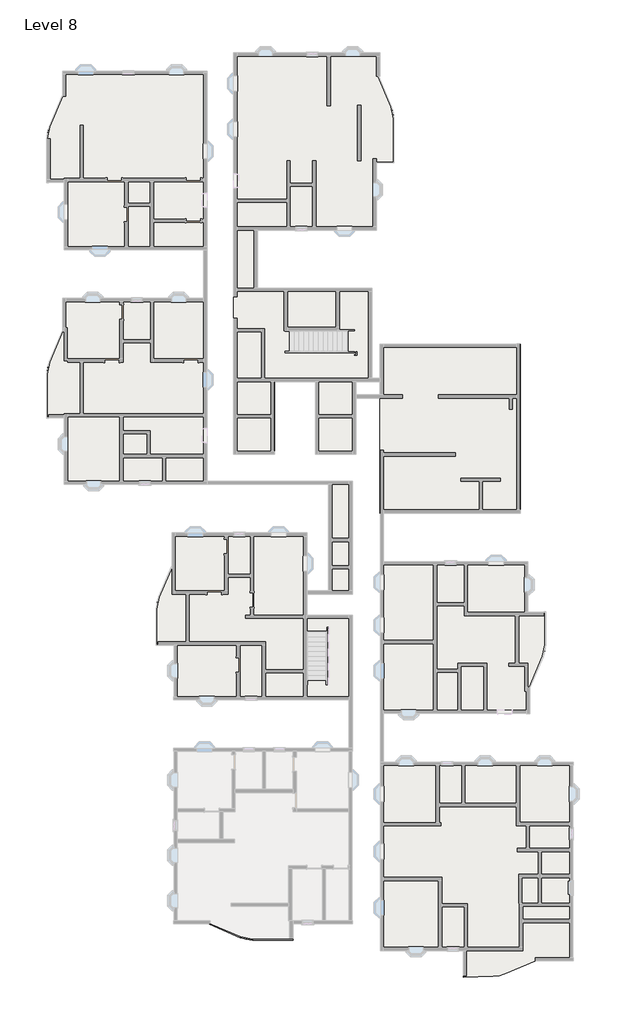
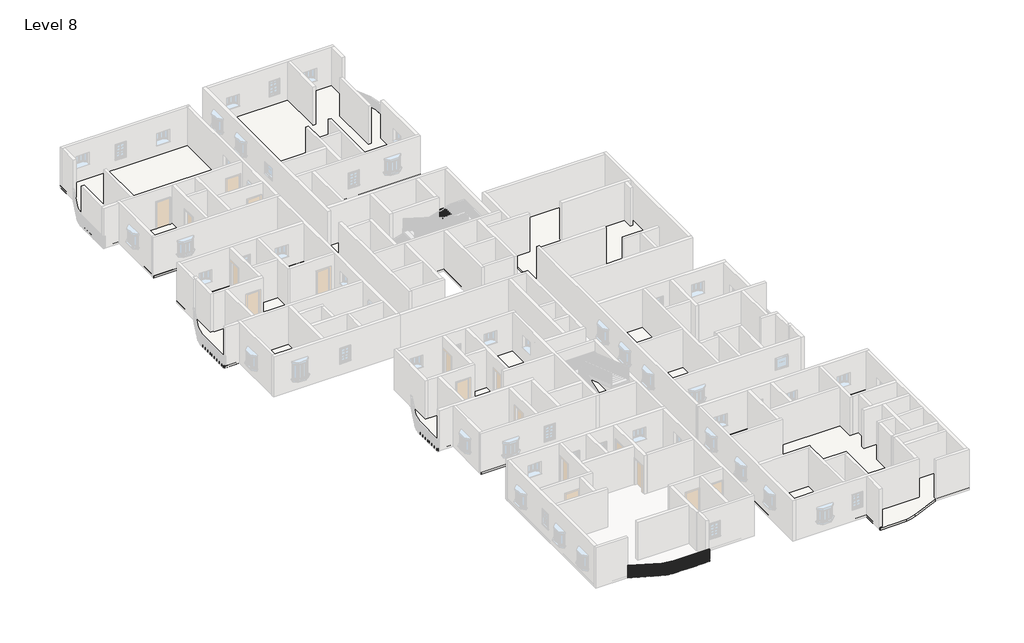
# One storey, part 5 of 14: 24 roofs, 1 railing.
"""IFC4 building model written with IfcOpenShell, lengths in millimetres."""

from ifc_helpers import new_model, si_unit, point, frame, frame_2d, origin, place, context, project, spatial, polyline, circle_curve, trimmed, segment, composite_curve, outline, extrude, element, save
from ifc_brep_helpers import plane_surface, cylinder_surface, revolved_surface, advanced_brep

model = new_model("IFC4")

# Units and contexts
model_context = context("Model", 3, world=origin())
ifc_project = project(units=[si_unit("LENGTHUNIT", "METRE", prefix="MILLI")], contexts=[model_context])

# Site, building, storey
site = spatial("IfcSite", under=ifc_project)
building = spatial("IfcBuilding", under=site)
storey = spatial("IfcBuildingStorey", under=building, Name="Level 8", Elevation=21336.0)

# Railing
placement = place(None, origin())
element("IfcRailing", 1, ObjectType="Handrail - Rectangular", at=placement, inside=storey, context=model_context, shape_type="SolidModel", body=[
    advanced_brep(
    [(-10014.8722294, -25076.9923935, 22250.4), (-10014.8722294, -25076.9923935, 22199.6), (-10034.8694485, -25123.6909077, 22199.6), (-10034.8694485, -25123.6909077, 22250.4), (-8065.5370278, -25911.7359335, 22250.4), (-8065.5370278, -25911.7359335, 22199.6), (-8085.5342469, -25958.4344477, 22199.6), (-8085.5342469, -25958.4344477, 22250.4), (-7315.6413127, -26065.5416506, 22199.6), (-7315.6413127, -26065.5416506, 22250.4), (-7315.6413127, -26116.3416506, 22199.6), (-7315.6413127, -26116.3416506, 22250.4), (-4746.0891351, -26065.5416506, 22250.4), (-4746.0891351, -26116.3416506, 22250.4), (-4746.0891351, -26116.3416506, 22199.6), (-4746.0891351, -26065.5416506, 22199.6)],
    [
        (0, 1),
        (1, 2),
        (2, 3),
        (3, 0),
        (0, 4),
        (4, 5),
        (5, 1),
        (5, 6),
        (6, 2),
        (6, 7),
        (7, 3),
        (7, 4),
        (8, 5, circle_curve(frame((-7315.6413127, -24160.5416506, 22199.6), z_axis=(0.0, 0.0, -1.0), x_axis=(-0.3936460446736572, -0.9192620907623599, 0.0)), 1905.0)),
        (4, 9, circle_curve(frame((-7315.6413127, -24160.5416506, 22250.4), z_axis=(0.0, 0.0, 1.0), x_axis=(-0.3936460446736572, -0.9192620907623599, 0.0)), 1905.0)),
        (9, 8),
        (10, 6, circle_curve(frame((-7315.6413127, -24160.5416506, 22199.6), z_axis=(0.0, 0.0, -1.0), x_axis=(-0.3936460446736572, -0.9192620907623599, 0.0)), 1955.8)),
        (8, 10),
        (11, 7, circle_curve(frame((-7315.6413127, -24160.5416506, 22250.4), z_axis=(0.0, 0.0, -1.0), x_axis=(-0.3936460446736572, -0.9192620907623599, 0.0)), 1955.8)),
        (10, 11),
        (11, 9),
        (12, 13),
        (13, 14),
        (14, 15),
        (15, 12),
        (9, 12),
        (15, 8),
        (14, 10),
        (13, 11),
    ],
    [
        plane_surface(frame((-10024.8708389, -25100.3416506, 22250.4), z_axis=(-0.9192620907623597, 0.39364604467365766, 0.0), x_axis=(0.39364604467365766, 0.9192620907623597, 0.0))),
        plane_surface(frame((-10014.8722294, -25076.9923935, 22250.4), z_axis=(0.3936460446736575, 0.9192620907623598, 0.0), x_axis=(0.9192620907623598, -0.3936460446736575, 0.0))),
        plane_surface(frame((-10014.8722294, -25076.9923935, 22199.6), z_axis=(0.0, 0.0, -1.0), x_axis=(0.9192620907623598, -0.3936460446736575, 0.0))),
        plane_surface(frame((-10034.8694485, -25123.6909077, 22199.6), z_axis=(-0.39364604467365766, -0.9192620907623597, 0.0), x_axis=(0.9192620907623597, -0.39364604467365766, 0.0))),
        plane_surface(frame((-10034.8694485, -25123.6909077, 22250.4), z_axis=(0.0, 0.0, 1.0), x_axis=(0.9192620907623597, -0.39364604467365766, 0.0))),
        revolved_surface(polyline([(-8065.537027803317, -25911.735933502296, 22250.4), (-8065.537027803317, -25911.735933502296, 22199.6)]), (-7315.6413127, -24160.5416506, 22250.4), (0.0, 0.0, 1.0)),
        plane_surface(frame((-7315.6413127, -24160.5416506, 22199.6), z_axis=(0.0, 0.0, -1.0), x_axis=(-0.3936460446736572, -0.9192620907623599, 0.0))),
        cylinder_surface(frame((-7315.6413127, -24160.5416506, 22250.4), z_axis=(0.0, 0.0, 1.0), x_axis=(-0.3936460446736572, -0.9192620907623599, 0.0)), 1955.8),
        plane_surface(frame((-7315.6413127, -24160.5416506, 22250.4), z_axis=(0.0, 0.0, 1.0), x_axis=(-0.3936460446736572, -0.9192620907623599, 0.0))),
        plane_surface(frame((-4746.0891351, -26090.9416506, 22250.4), z_axis=(1.0, 0.0, 0.0), x_axis=(0.0, 1.0, 0.0))),
        plane_surface(frame((-7315.6413127, -26065.5416506, 22250.4), z_axis=(0.0, 1.0, 0.0), x_axis=(1.0, 0.0, 0.0))),
        plane_surface(frame((-7315.6413127, -26065.5416506, 22199.6), z_axis=(0.0, 0.0, -1.0), x_axis=(1.0, 0.0, 0.0))),
        plane_surface(frame((-7315.6413127, -26116.3416506, 22199.6), z_axis=(0.0, -1.0, 0.0), x_axis=(1.0, 0.0, 0.0))),
        plane_surface(frame((-7315.6413127, -26116.3416506, 22250.4), z_axis=(0.0, 0.0, 1.0), x_axis=(1.0, 0.0, 0.0))),
    ],
    [
        (0, [[1, 2, 3, 4]]),
        (1, [[-1, 5, 6, 7]]),
        (2, [[-2, -7, 8, 9]]),
        (3, [[-3, -9, 10, 11]]),
        (4, [[-4, -11, 12, -5]]),
        (5, [[13, -6, 14, 15]]),
        (6, [[16, -8, -13, 17]]),
        (7, [[18, -10, -16, 19]]),
        (8, [[-14, -12, -18, 20]]),
        (9, [[21, 22, 23, 24]]),
        (10, [[-15, 25, -24, 26]]),
        (11, [[-17, -26, -23, 27]]),
        (12, [[-19, -27, -22, 28]]),
        (13, [[-20, -28, -21, -25]]),
    ],
),
    extrude(outline(polyline([(-4785.1663127, -26100.4666506), (-4785.1663127, -26081.4166506), (-4766.1163127, -26081.4166506), (-4766.1163127, -26100.4666506), (-4785.1663127, -26100.4666506)])), frame((0.0, 0.0, 21336.0), z_axis=(0.0, 0.0, 1.0), x_axis=(1.0, 0.0, 0.0)), (0.0, 0.0, 1.0), 863.6),
    extrude(outline(polyline([(-4886.7663127, -26100.4666506), (-4886.7663127, -26081.4166506), (-4867.7163127, -26081.4166506), (-4867.7163127, -26100.4666506), (-4886.7663127, -26100.4666506)])), frame((0.0, 0.0, 21336.0), z_axis=(0.0, 0.0, 1.0), x_axis=(1.0, 0.0, 0.0)), (0.0, 0.0, 1.0), 863.6),
    extrude(outline(polyline([(-4988.3663127, -26100.4666506), (-4988.3663127, -26081.4166506), (-4969.3163127, -26081.4166506), (-4969.3163127, -26100.4666506), (-4988.3663127, -26100.4666506)])), frame((0.0, 0.0, 21336.0), z_axis=(0.0, 0.0, 1.0), x_axis=(1.0, 0.0, 0.0)), (0.0, 0.0, 1.0), 863.6),
    extrude(outline(polyline([(-5089.9663127, -26100.4666506), (-5089.9663127, -26081.4166506), (-5070.9163127, -26081.4166506), (-5070.9163127, -26100.4666506), (-5089.9663127, -26100.4666506)])), frame((0.0, 0.0, 21336.0), z_axis=(0.0, 0.0, 1.0), x_axis=(1.0, 0.0, 0.0)), (0.0, 0.0, 1.0), 863.6),
    extrude(outline(polyline([(-5191.5663127, -26100.4666506), (-5191.5663127, -26081.4166506), (-5172.5163127, -26081.4166506), (-5172.5163127, -26100.4666506), (-5191.5663127, -26100.4666506)])), frame((0.0, 0.0, 21336.0), z_axis=(0.0, 0.0, 1.0), x_axis=(1.0, 0.0, 0.0)), (0.0, 0.0, 1.0), 863.6),
    extrude(outline(polyline([(-5293.1663127, -26100.4666506), (-5293.1663127, -26081.4166506), (-5274.1163127, -26081.4166506), (-5274.1163127, -26100.4666506), (-5293.1663127, -26100.4666506)])), frame((0.0, 0.0, 21336.0), z_axis=(0.0, 0.0, 1.0), x_axis=(1.0, 0.0, 0.0)), (0.0, 0.0, 1.0), 863.6),
    extrude(outline(polyline([(-5394.7663127, -26100.4666506), (-5394.7663127, -26081.4166506), (-5375.7163127, -26081.4166506), (-5375.7163127, -26100.4666506), (-5394.7663127, -26100.4666506)])), frame((0.0, 0.0, 21336.0), z_axis=(0.0, 0.0, 1.0), x_axis=(1.0, 0.0, 0.0)), (0.0, 0.0, 1.0), 863.6),
    extrude(outline(polyline([(-5496.3663127, -26100.4666506), (-5496.3663127, -26081.4166506), (-5477.3163127, -26081.4166506), (-5477.3163127, -26100.4666506), (-5496.3663127, -26100.4666506)])), frame((0.0, 0.0, 21336.0), z_axis=(0.0, 0.0, 1.0), x_axis=(1.0, 0.0, 0.0)), (0.0, 0.0, 1.0), 863.6),
    extrude(outline(polyline([(-5597.9663127, -26100.4666506), (-5597.9663127, -26081.4166506), (-5578.9163127, -26081.4166506), (-5578.9163127, -26100.4666506), (-5597.9663127, -26100.4666506)])), frame((0.0, 0.0, 21336.0), z_axis=(0.0, 0.0, 1.0), x_axis=(1.0, 0.0, 0.0)), (0.0, 0.0, 1.0), 863.6),
    extrude(outline(polyline([(-5699.5663127, -26100.4666506), (-5699.5663127, -26081.4166506), (-5680.5163127, -26081.4166506), (-5680.5163127, -26100.4666506), (-5699.5663127, -26100.4666506)])), frame((0.0, 0.0, 21336.0), z_axis=(0.0, 0.0, 1.0), x_axis=(1.0, 0.0, 0.0)), (0.0, 0.0, 1.0), 863.6),
    extrude(outline(polyline([(-5801.1663127, -26100.4666506), (-5801.1663127, -26081.4166506), (-5782.1163127, -26081.4166506), (-5782.1163127, -26100.4666506), (-5801.1663127, -26100.4666506)])), frame((0.0, 0.0, 21336.0), z_axis=(0.0, 0.0, 1.0), x_axis=(1.0, 0.0, 0.0)), (0.0, 0.0, 1.0), 863.6),
    extrude(outline(polyline([(-5902.7663127, -26100.4666506), (-5902.7663127, -26081.4166506), (-5883.7163127, -26081.4166506), (-5883.7163127, -26100.4666506), (-5902.7663127, -26100.4666506)])), frame((0.0, 0.0, 21336.0), z_axis=(0.0, 0.0, 1.0), x_axis=(1.0, 0.0, 0.0)), (0.0, 0.0, 1.0), 863.6),
    extrude(outline(polyline([(-6004.3663127, -26100.4666506), (-6004.3663127, -26081.4166506), (-5985.3163127, -26081.4166506), (-5985.3163127, -26100.4666506), (-6004.3663127, -26100.4666506)])), frame((0.0, 0.0, 21336.0), z_axis=(0.0, 0.0, 1.0), x_axis=(1.0, 0.0, 0.0)), (0.0, 0.0, 1.0), 863.6),
    extrude(outline(polyline([(-6105.9663127, -26100.4666506), (-6105.9663127, -26081.4166506), (-6086.9163127, -26081.4166506), (-6086.9163127, -26100.4666506), (-6105.9663127, -26100.4666506)])), frame((0.0, 0.0, 21336.0), z_axis=(0.0, 0.0, 1.0), x_axis=(1.0, 0.0, 0.0)), (0.0, 0.0, 1.0), 863.6),
    extrude(outline(polyline([(-6207.5663127, -26100.4666506), (-6207.5663127, -26081.4166506), (-6188.5163127, -26081.4166506), (-6188.5163127, -26100.4666506), (-6207.5663127, -26100.4666506)])), frame((0.0, 0.0, 21336.0), z_axis=(0.0, 0.0, 1.0), x_axis=(1.0, 0.0, 0.0)), (0.0, 0.0, 1.0), 863.6),
    extrude(outline(polyline([(-6309.1663127, -26100.4666506), (-6309.1663127, -26081.4166506), (-6290.1163127, -26081.4166506), (-6290.1163127, -26100.4666506), (-6309.1663127, -26100.4666506)])), frame((0.0, 0.0, 21336.0), z_axis=(0.0, 0.0, 1.0), x_axis=(1.0, 0.0, 0.0)), (0.0, 0.0, 1.0), 863.6),
    extrude(outline(polyline([(-6410.7663127, -26100.4666506), (-6410.7663127, -26081.4166506), (-6391.7163127, -26081.4166506), (-6391.7163127, -26100.4666506), (-6410.7663127, -26100.4666506)])), frame((0.0, 0.0, 21336.0), z_axis=(0.0, 0.0, 1.0), x_axis=(1.0, 0.0, 0.0)), (0.0, 0.0, 1.0), 863.6),
    extrude(outline(polyline([(-6512.3663127, -26100.4666506), (-6512.3663127, -26081.4166506), (-6493.3163127, -26081.4166506), (-6493.3163127, -26100.4666506), (-6512.3663127, -26100.4666506)])), frame((0.0, 0.0, 21336.0), z_axis=(0.0, 0.0, 1.0), x_axis=(1.0, 0.0, 0.0)), (0.0, 0.0, 1.0), 863.6),
    extrude(outline(polyline([(-6613.9663127, -26100.4666506), (-6613.9663127, -26081.4166506), (-6594.9163127, -26081.4166506), (-6594.9163127, -26100.4666506), (-6613.9663127, -26100.4666506)])), frame((0.0, 0.0, 21336.0), z_axis=(0.0, 0.0, 1.0), x_axis=(1.0, 0.0, 0.0)), (0.0, 0.0, 1.0), 863.6),
    extrude(outline(polyline([(-6715.5663127, -26100.4666506), (-6715.5663127, -26081.4166506), (-6696.5163127, -26081.4166506), (-6696.5163127, -26100.4666506), (-6715.5663127, -26100.4666506)])), frame((0.0, 0.0, 21336.0), z_axis=(0.0, 0.0, 1.0), x_axis=(1.0, 0.0, 0.0)), (0.0, 0.0, 1.0), 863.6),
    extrude(outline(polyline([(-6817.1663127, -26100.4666506), (-6817.1663127, -26081.4166506), (-6798.1163127, -26081.4166506), (-6798.1163127, -26100.4666506), (-6817.1663127, -26100.4666506)])), frame((0.0, 0.0, 21336.0), z_axis=(0.0, 0.0, 1.0), x_axis=(1.0, 0.0, 0.0)), (0.0, 0.0, 1.0), 863.6),
    extrude(outline(polyline([(-6918.7663127, -26100.4666506), (-6918.7663127, -26081.4166506), (-6899.7163127, -26081.4166506), (-6899.7163127, -26100.4666506), (-6918.7663127, -26100.4666506)])), frame((0.0, 0.0, 21336.0), z_axis=(0.0, 0.0, 1.0), x_axis=(1.0, 0.0, 0.0)), (0.0, 0.0, 1.0), 863.6),
    extrude(outline(polyline([(-7020.3663127, -26100.4666506), (-7020.3663127, -26081.4166506), (-7001.3163127, -26081.4166506), (-7001.3163127, -26100.4666506), (-7020.3663127, -26100.4666506)])), frame((0.0, 0.0, 21336.0), z_axis=(0.0, 0.0, 1.0), x_axis=(1.0, 0.0, 0.0)), (0.0, 0.0, 1.0), 863.6),
    extrude(outline(polyline([(-7121.9663127, -26100.4666506), (-7121.9663127, -26081.4166506), (-7102.9163127, -26081.4166506), (-7102.9163127, -26100.4666506), (-7121.9663127, -26100.4666506)])), frame((0.0, 0.0, 21336.0), z_axis=(0.0, 0.0, 1.0), x_axis=(1.0, 0.0, 0.0)), (0.0, 0.0, 1.0), 863.6),
    extrude(outline(polyline([(-7223.5663127, -26100.4666506), (-7223.5663127, -26081.4166506), (-7204.5163127, -26081.4166506), (-7204.5163127, -26100.4666506), (-7223.5663127, -26100.4666506)])), frame((0.0, 0.0, 21336.0), z_axis=(0.0, 0.0, 1.0), x_axis=(1.0, 0.0, 0.0)), (0.0, 0.0, 1.0), 863.6),
    extrude(outline(polyline([(-7395.3185803, -26098.8530973), (-7394.6296262, -26079.8155596), (-7375.5920885, -26080.5045137), (-7376.2810426, -26099.5420514), (-7395.3185803, -26098.8530973)])), frame((0.0, 0.0, 21336.0), z_axis=(0.0, 0.0, 1.0), x_axis=(1.0, 0.0, 0.0)), (0.0, 0.0, 1.0), 863.6),
    extrude(outline(polyline([(-7497.177549, -26091.9774704), (-7495.4880357, -26073.0025384), (-7476.5131037, -26074.6920517), (-7478.2026169, -26093.6669837), (-7497.177549, -26091.9774704)])), frame((0.0, 0.0, 21336.0), z_axis=(0.0, 0.0, 1.0), x_axis=(1.0, 0.0, 0.0)), (0.0, 0.0, 1.0), 863.6),
    extrude(outline(polyline([(-7598.5337632, -26079.7528408), (-7595.8483698, -26060.8930645), (-7576.9885935, -26063.5784579), (-7579.6739869, -26082.4382342), (-7598.5337632, -26079.7528408)])), frame((0.0, 0.0, 21336.0), z_axis=(0.0, 0.0, 1.0), x_axis=(1.0, 0.0, 0.0)), (0.0, 0.0, 1.0), 863.6),
    extrude(outline(polyline([(-7699.1065227, -26062.2130639), (-7695.4326862, -26043.5206744), (-7676.7402967, -26047.1945108), (-7680.4141332, -26065.8869003), (-7699.1065227, -26062.2130639)])), frame((0.0, 0.0, 21336.0), z_axis=(0.0, 0.0, 1.0), x_axis=(1.0, 0.0, 0.0)), (0.0, 0.0, 1.0), 863.6),
    extrude(outline(polyline([(-7798.6172969, -26039.4067149), (-7793.9651918, -26020.9334797), (-7775.4919566, -26025.5855848), (-7780.1440617, -26044.05882), (-7798.6172969, -26039.4067149)])), frame((0.0, 0.0, 21336.0), z_axis=(0.0, 0.0, 1.0), x_axis=(1.0, 0.0, 0.0)), (0.0, 0.0, 1.0), 863.6),
    extrude(outline(polyline([(-7896.7904963, -26011.396955), (-7891.1730064, -25993.1940347), (-7872.9700861, -25998.8115246), (-7878.587576, -26017.0144449), (-7896.7904963, -26011.396955)])), frame((0.0, 0.0, 21336.0), z_axis=(0.0, 0.0, 1.0), x_axis=(1.0, 0.0, 0.0)), (0.0, 0.0, 1.0), 863.6),
    extrude(outline(polyline([(-7993.3542357, -25978.2613554), (-7986.7869183, -25960.379162), (-7968.9047249, -25966.9464794), (-7975.4720423, -25984.8286729), (-7993.3542357, -25978.2613554)])), frame((0.0, 0.0, 21336.0), z_axis=(0.0, 0.0, 1.0), x_axis=(1.0, 0.0, 0.0)), (0.0, 0.0, 1.0), 863.6),
    extrude(outline(polyline([(-8169.4357205, -25905.2369062), (-8161.9367633, -25887.7249634), (-8144.4248205, -25895.2239205), (-8151.9237777, -25912.7358634), (-8169.4357205, -25905.2369062)])), frame((0.0, 0.0, 21336.0), z_axis=(0.0, 0.0, 1.0), x_axis=(1.0, 0.0, 0.0)), (0.0, 0.0, 1.0), 863.6),
    extrude(outline(polyline([(-8262.8327489, -25865.2424681), (-8255.3337918, -25847.7305252), (-8237.8218489, -25855.2294824), (-8245.3208061, -25872.7414252), (-8262.8327489, -25865.2424681)])), frame((0.0, 0.0, 21336.0), z_axis=(0.0, 0.0, 1.0), x_axis=(1.0, 0.0, 0.0)), (0.0, 0.0, 1.0), 863.6),
    extrude(outline(polyline([(-8356.2297773, -25825.2480299), (-8348.7308202, -25807.7360871), (-8331.2188774, -25815.2350443), (-8338.7178345, -25832.7469871), (-8356.2297773, -25825.2480299)])), frame((0.0, 0.0, 21336.0), z_axis=(0.0, 0.0, 1.0), x_axis=(1.0, 0.0, 0.0)), (0.0, 0.0, 1.0), 863.6),
    extrude(outline(polyline([(-8449.6268058, -25785.2535918), (-8442.1278486, -25767.741649), (-8424.6159058, -25775.2406061), (-8432.1148629, -25792.752549), (-8449.6268058, -25785.2535918)])), frame((0.0, 0.0, 21336.0), z_axis=(0.0, 0.0, 1.0), x_axis=(1.0, 0.0, 0.0)), (0.0, 0.0, 1.0), 863.6),
    extrude(outline(polyline([(-8543.0238342, -25745.2591537), (-8535.524877, -25727.7472108), (-8518.0129342, -25735.246168), (-8525.5118914, -25752.7581108), (-8543.0238342, -25745.2591537)])), frame((0.0, 0.0, 21336.0), z_axis=(0.0, 0.0, 1.0), x_axis=(1.0, 0.0, 0.0)), (0.0, 0.0, 1.0), 863.6),
    extrude(outline(polyline([(-8636.4208626, -25705.2647155), (-8628.9219055, -25687.7527727), (-8611.4099626, -25695.2517298), (-8618.9089198, -25712.7636727), (-8636.4208626, -25705.2647155)])), frame((0.0, 0.0, 21336.0), z_axis=(0.0, 0.0, 1.0), x_axis=(1.0, 0.0, 0.0)), (0.0, 0.0, 1.0), 863.6),
    extrude(outline(polyline([(-8729.817891, -25665.2702774), (-8722.3189339, -25647.7583346), (-8704.806991, -25655.2572917), (-8712.3059482, -25672.7692345), (-8729.817891, -25665.2702774)])), frame((0.0, 0.0, 21336.0), z_axis=(0.0, 0.0, 1.0), x_axis=(1.0, 0.0, 0.0)), (0.0, 0.0, 1.0), 863.6),
    extrude(outline(polyline([(-8823.2149194, -25625.2758392), (-8815.7159623, -25607.7638964), (-8798.2040195, -25615.2628536), (-8805.7029766, -25632.7747964), (-8823.2149194, -25625.2758392)])), frame((0.0, 0.0, 21336.0), z_axis=(0.0, 0.0, 1.0), x_axis=(1.0, 0.0, 0.0)), (0.0, 0.0, 1.0), 863.6),
    extrude(outline(polyline([(-8916.6119479, -25585.2814011), (-8909.1129907, -25567.7694583), (-8891.6010479, -25575.2684154), (-8899.100005, -25592.7803583), (-8916.6119479, -25585.2814011)])), frame((0.0, 0.0, 21336.0), z_axis=(0.0, 0.0, 1.0), x_axis=(1.0, 0.0, 0.0)), (0.0, 0.0, 1.0), 863.6),
    extrude(outline(polyline([(-9010.0089763, -25545.286963), (-9002.5100191, -25527.7750201), (-8984.9980763, -25535.2739773), (-8992.4970335, -25552.7859201), (-9010.0089763, -25545.286963)])), frame((0.0, 0.0, 21336.0), z_axis=(0.0, 0.0, 1.0), x_axis=(1.0, 0.0, 0.0)), (0.0, 0.0, 1.0), 863.6),
    extrude(outline(polyline([(-9103.4060047, -25505.2925248), (-9095.9070476, -25487.780582), (-9078.3951047, -25495.2795391), (-9085.8940619, -25512.791482), (-9103.4060047, -25505.2925248)])), frame((0.0, 0.0, 21336.0), z_axis=(0.0, 0.0, 1.0), x_axis=(1.0, 0.0, 0.0)), (0.0, 0.0, 1.0), 863.6),
    extrude(outline(polyline([(-9196.8030331, -25465.2980867), (-9189.304076, -25447.7861439), (-9171.7921332, -25455.285101), (-9179.2910903, -25472.7970438), (-9196.8030331, -25465.2980867)])), frame((0.0, 0.0, 21336.0), z_axis=(0.0, 0.0, 1.0), x_axis=(1.0, 0.0, 0.0)), (0.0, 0.0, 1.0), 863.6),
    extrude(outline(polyline([(-9290.2000616, -25425.3036485), (-9282.7011044, -25407.7917057), (-9265.1891616, -25415.2906629), (-9272.6881187, -25432.8026057), (-9290.2000616, -25425.3036485)])), frame((0.0, 0.0, 21336.0), z_axis=(0.0, 0.0, 1.0), x_axis=(1.0, 0.0, 0.0)), (0.0, 0.0, 1.0), 863.6),
    extrude(outline(polyline([(-9383.59709, -25385.3092104), (-9376.0981328, -25367.7972676), (-9358.58619, -25375.2962247), (-9366.0851471, -25392.8081676), (-9383.59709, -25385.3092104)])), frame((0.0, 0.0, 21336.0), z_axis=(0.0, 0.0, 1.0), x_axis=(1.0, 0.0, 0.0)), (0.0, 0.0, 1.0), 863.6),
    extrude(outline(polyline([(-9476.9941184, -25345.3147723), (-9469.4951612, -25327.8028294), (-9451.9832184, -25335.3017866), (-9459.4821756, -25352.8137294), (-9476.9941184, -25345.3147723)])), frame((0.0, 0.0, 21336.0), z_axis=(0.0, 0.0, 1.0), x_axis=(1.0, 0.0, 0.0)), (0.0, 0.0, 1.0), 863.6),
    extrude(outline(polyline([(-9570.3911468, -25305.3203341), (-9562.8921897, -25287.8083913), (-9545.3802468, -25295.3073485), (-9552.879204, -25312.8192913), (-9570.3911468, -25305.3203341)])), frame((0.0, 0.0, 21336.0), z_axis=(0.0, 0.0, 1.0), x_axis=(1.0, 0.0, 0.0)), (0.0, 0.0, 1.0), 863.6),
    extrude(outline(polyline([(-9663.7881752, -25265.325896), (-9656.2892181, -25247.8139532), (-9638.7772753, -25255.3129103), (-9646.2762324, -25272.8248531), (-9663.7881752, -25265.325896)])), frame((0.0, 0.0, 21336.0), z_axis=(0.0, 0.0, 1.0), x_axis=(1.0, 0.0, 0.0)), (0.0, 0.0, 1.0), 863.6),
    extrude(outline(polyline([(-9757.1852037, -25225.3314579), (-9749.6862465, -25207.819515), (-9732.1743037, -25215.3184722), (-9739.6732608, -25232.830415), (-9757.1852037, -25225.3314579)])), frame((0.0, 0.0, 21336.0), z_axis=(0.0, 0.0, 1.0), x_axis=(1.0, 0.0, 0.0)), (0.0, 0.0, 1.0), 863.6),
    extrude(outline(polyline([(-9850.5822321, -25185.3370197), (-9843.0832749, -25167.8250769), (-9825.5713321, -25175.324034), (-9833.0702893, -25192.8359769), (-9850.5822321, -25185.3370197)])), frame((0.0, 0.0, 21336.0), z_axis=(0.0, 0.0, 1.0), x_axis=(1.0, 0.0, 0.0)), (0.0, 0.0, 1.0), 863.6),
    extrude(outline(polyline([(-9943.9792605, -25145.3425816), (-9936.4803034, -25127.8306387), (-9918.9683605, -25135.3295959), (-9926.4673177, -25152.8415387), (-9943.9792605, -25145.3425816)])), frame((0.0, 0.0, 21336.0), z_axis=(0.0, 0.0, 1.0), x_axis=(1.0, 0.0, 0.0)), (0.0, 0.0, 1.0), 863.6),
    extrude(outline(polyline([(-7325.1663127, -26100.4666506), (-7325.1663127, -26081.4166506), (-7306.1163127, -26081.4166506), (-7306.1163127, -26100.4666506), (-7325.1663127, -26100.4666506)])), frame((0.0, 0.0, 21336.0), z_axis=(0.0, 0.0, 1.0), x_axis=(1.0, 0.0, 0.0)), (0.0, 0.0, 1.0), 863.6),
    extrude(outline(polyline([(-8088.0410874, -25940.0916834), (-8080.5421302, -25922.5797406), (-8063.0301874, -25930.0786978), (-8070.5291445, -25947.5906406), (-8088.0410874, -25940.0916834)])), frame((0.0, 0.0, 21336.0), z_axis=(0.0, 0.0, 1.0), x_axis=(1.0, 0.0, 0.0)), (0.0, 0.0, 1.0), 863.6),
    extrude(outline(polyline([(-4765.1391351, -26100.4666506), (-4765.1391351, -26081.4166506), (-4746.0891351, -26081.4166506), (-4746.0891351, -26100.4666506), (-4765.1391351, -26100.4666506)])), frame((0.0, 0.0, 21336.0), z_axis=(0.0, 0.0, 1.0), x_axis=(1.0, 0.0, 0.0)), (0.0, 0.0, 1.0), 863.6),
    extrude(outline(polyline([(-10028.6203175, -25109.097622), (-10021.1213604, -25091.5856792), (-10003.6094175, -25099.0846363), (-10011.1083747, -25116.5965792), (-10028.6203175, -25109.097622)])), frame((0.0, 0.0, 21336.0), z_axis=(0.0, 0.0, 1.0), x_axis=(1.0, 0.0, 0.0)), (0.0, 0.0, 1.0), 863.6),
])

# Roofs
element("IfcRoof", 2, ObjectType="Generic - 12\"", at=placement, inside=storey, context=model_context, shape_type="SweptSolid", body=[
    extrude(outline(composite_curve([segment(polyline([(6070.4380523, -26783.9042694), (812.6380523, -26783.9042694), (812.6380523, -14845.9042694), (13017.3380523, -14845.9042694), (13017.3380523, -27431.6042694), (10660.5280667, -27431.6042694), (8711.1928652, -28266.3478094)]), True, "CONTINUOUS"), segment(trimmed(circle_curve(frame_2d((7951.2985405, -26491.8042694)), 1930.4), [point((8711.1928652, -28266.3478094))], [point((7953.0959373, -28422.2034326))], False, "CARTESIAN"), True, "CONTINUOUS"), segment(polyline([(7953.0959373, -28422.2034326), (6070.4380523, -28487.9472947), (6070.4380523, -26783.9042694)]), True, "CONTINUOUS")], self_intersect=False)), frame((0.0, 0.0, 21336.0), z_axis=(0.0, 0.0, 1.0), x_axis=(1.0, 0.0, 0.0)), (0.0, 0.0, 1.0), 152.4),
])
element("IfcRoof", 3, ObjectType="Generic - 12\"", at=placement, inside=storey, context=model_context, shape_type="SweptSolid", body=[
    extrude(outline(composite_curve([segment(polyline([(10274.1380523, -11759.8042694), (803.8108649, -11759.8042694), (803.8108649, -2133.2042694), (10159.8380523, -2133.2042694), (10159.8380523, -5352.6542694), (11264.7380523, -5352.6542694), (11264.7380523, -7397.5810633)]), True, "CONTINUOUS"), segment(trimmed(circle_curve(frame_2d((9334.3380523, -7397.5810633)), 1930.4), [point((11264.7380523, -7397.5810633))], [point((11108.8815923, -8157.475388))], False, "CARTESIAN"), True, "CONTINUOUS"), segment(polyline([(11108.8815923, -8157.475388), (10274.1380523, -10106.8105895), (10274.1380523, -11759.8042694)]), True, "CONTINUOUS")], self_intersect=False)), frame((0.0, 0.0, 21336.0), z_axis=(0.0, 0.0, 1.0), x_axis=(1.0, 0.0, 0.0)), (0.0, 0.0, 1.0), 152.4),
])
element("IfcRoof", 4, ObjectType="Generic - 12\"", at=placement, inside=storey, context=model_context, shape_type="SweptSolid", body=[
    extrude(outline(composite_curve([segment(polyline([(-13395.387215, -7421.9416506), (-13395.387215, -5140.4900045)]), True, "CONTINUOUS"), segment(trimmed(circle_curve(frame_2d((-11464.987215, -5140.4900045)), 1930.4), [point((-13395.387215, -5140.4900045))], [point((-13239.530755, -4380.5956799))], False, "CARTESIAN"), True, "CONTINUOUS"), segment(polyline([(-13239.530755, -4380.5956799), (-12404.787215, -2431.2604783), (-12404.787215, -322.6416506), (-3857.687215, -322.6416506), (-3857.687215, -5523.2916506), (-974.1891351, -5523.2916506), (-974.1891351, -10889.0416506), (-12290.487215, -10889.0416506), (-12290.487215, -7421.9416506), (-13395.387215, -7421.9416506)]), True, "CONTINUOUS")], self_intersect=False)), frame((0.0, 0.0, 21336.0), z_axis=(0.0, 0.0, 1.0), x_axis=(1.0, 0.0, 0.0)), (0.0, 0.0, 1.0), 152.4),
])
element("IfcRoof", 5, ObjectType="Generic - 12\"", at=placement, inside=storey, context=model_context, shape_type="SweptSolid", body=[
    extrude(outline(polyline([(-2472.7891351, 2953.9583494), (-961.4891351, 2953.9583494), (-961.4891351, -4202.4916506), (-2472.7891351, -4202.4916506), (-2472.7891351, 2953.9583494)])), frame((0.0, 0.0, 21336.0), z_axis=(0.0, 0.0, 1.0), x_axis=(1.0, 0.0, 0.0)), (0.0, 0.0, 1.0), 152.4),
])
element("IfcRoof", 6, ObjectType="Generic - 12\"", at=placement, inside=storey, context=model_context, shape_type="SweptSolid", body=[
    extrude(outline(composite_curve([segment(polyline([(-10194.3891351, 2750.7583494), (-19236.7891351, 2750.7583494), (-19236.7891351, 6979.8583494), (-20341.6891351, 6979.8583494), (-20341.6891351, 9746.7948172)]), True, "CONTINUOUS"), segment(trimmed(circle_curve(frame_2d((-18411.2891351, 9746.7948172)), 1930.4), [point((-20341.6891351, 9746.7948172))], [point((-20185.8326751, 10506.6891419))], False, "CARTESIAN"), True, "CONTINUOUS"), segment(polyline([(-20185.8326751, 10506.6891419), (-19351.0891351, 12456.0243434), (-19351.0891351, 14536.3583494), (-10194.3891351, 14536.3583494), (-10194.3891351, 2750.7583494)]), True, "CONTINUOUS")], self_intersect=False)), frame((0.0, 0.0, 21336.0), z_axis=(0.0, 0.0, 1.0), x_axis=(1.0, 0.0, 0.0)), (0.0, 0.0, 1.0), 152.4),
])
element("IfcRoof", 7, ObjectType="Generic - 12\"", at=placement, inside=storey, context=model_context, shape_type="SweptSolid", body=[
    extrude(outline(composite_curve([segment(polyline([(-10194.3891351, 17609.7583494), (-19236.7891351, 17609.7583494), (-19236.7891351, 21889.6583494), (-20341.6891351, 21889.6583494), (-20341.6891351, 24656.5948172)]), True, "CONTINUOUS"), segment(trimmed(circle_curve(frame_2d((-18411.2891351, 24656.5948172)), 1930.4), [point((-20341.6891351, 24656.5948172))], [point((-20185.8326751, 25416.4891419))], False, "CARTESIAN"), True, "CONTINUOUS"), segment(polyline([(-20185.8326751, 25416.4891419), (-19351.0891351, 27365.8243434), (-19351.0891351, 28950.8583494), (-10194.3891351, 28950.8583494), (-10194.3891351, 17609.7583494)]), True, "CONTINUOUS")], self_intersect=False)), frame((0.0, 0.0, 21336.0), z_axis=(0.0, 0.0, 1.0), x_axis=(1.0, 0.0, 0.0)), (0.0, 0.0, 1.0), 152.4),
])
element("IfcRoof", 8, ObjectType="Generic - 12\"", at=placement, inside=storey, context=model_context, shape_type="SweptSolid", body=[
    extrude(outline(composite_curve([segment(polyline([(-8492.5891351, 18875.1215905), (-8492.5891351, 30101.9215905), (664.1108649, 30101.9215905), (664.1108649, 28631.1875845), (1498.8544049, 26681.8523829)]), True, "CONTINUOUS"), segment(trimmed(circle_curve(frame_2d((-275.6891351, 25921.9580583)), 1930.4), [point((1498.8544049, 26681.8523829))], [point((1654.7108649, 25921.9580583))], False, "CARTESIAN"), True, "CONTINUOUS"), segment(polyline([(1654.7108649, 25921.9580583), (1654.7108649, 23155.0215905), (549.8108649, 23155.0215905), (549.8108649, 18875.1215905), (-8492.5891351, 18875.1215905)]), True, "CONTINUOUS")], self_intersect=False)), frame((0.0, 0.0, 21336.0), z_axis=(0.0, 0.0, 1.0), x_axis=(1.0, 0.0, 0.0)), (0.0, 0.0, 1.0), 152.4),
])
element("IfcRoof", 9, ObjectType="Generic - 12\"", at=placement, inside=storey, context=model_context, shape_type="SweptSolid", body=[
    extrude(outline(polyline([(-8492.5891351, 9478.4949943), (-5914.4891351, 9478.4949943), (-5914.4891351, 4665.1949943), (-8492.5891351, 4665.1949943), (-8492.5891351, 9478.4949943)])), frame((0.0, 0.0, 21336.0), z_axis=(0.0, 0.0, 1.0), x_axis=(1.0, 0.0, 0.0)), (0.0, 0.0, 1.0), 152.4),
])
element("IfcRoof", 10, ObjectType="Generic - 12\"", at=placement, inside=storey, context=model_context, shape_type="SweptSolid", body=[
    extrude(outline(polyline([(-3310.9891351, 9478.4949943), (-745.5891351, 9478.4949943), (-745.5891351, 4652.4949943), (-3310.9891351, 4652.4949943), (-3310.9891351, 9478.4949943)])), frame((0.0, 0.0, 21336.0), z_axis=(0.0, 0.0, 1.0), x_axis=(1.0, 0.0, 0.0)), (0.0, 0.0, 1.0), 152.4),
])
element("IfcRoof", 11, ObjectType="Generic - 12\"", at=placement, inside=storey, context=model_context, shape_type="SweptSolid", body=[
    extrude(outline(polyline([(-8492.5891351, 19078.3215905), (-6993.9891351, 19078.3215905), (-6993.9891351, 14988.9215905), (-8492.5891351, 14988.9215905), (-8492.5891351, 19078.3215905)])), frame((0.0, 0.0, 21336.0), z_axis=(0.0, 0.0, 1.0), x_axis=(1.0, 0.0, 0.0)), (0.0, 0.0, 1.0), 152.4),
])
element("IfcRoof", 12, ObjectType="Generic - 12\"", at=placement, inside=storey, context=model_context, shape_type="SweptSolid", body=[
    extrude(outline(polyline([(-8492.5891351, 15192.1215905), (257.7108649, 15192.1215905), (257.7108649, 9275.2949943), (-8492.5891351, 9275.2949943), (-8492.5891351, 15192.1215905)])), frame((0.0, 0.0, 21336.0), z_axis=(0.0, 0.0, 1.0), x_axis=(1.0, 0.0, 0.0)), (0.0, 0.0, 1.0), 152.4),
])
element("IfcRoof", 13, ObjectType="Generic - 12\"", at=placement, inside=storey, context=model_context, shape_type="SweptSolid", body=[
    extrude(outline(polyline([(793.5880523, 11646.2957306), (9677.2380523, 11646.2957306), (9677.2380523, 940.1957306), (793.5880523, 940.1957306), (793.5880523, 11646.2957306)])), frame((0.0, 0.0, 21336.0), z_axis=(0.0, 0.0, 1.0), x_axis=(1.0, 0.0, 0.0)), (0.0, 0.0, 1.0), 152.4),
])
element("IfcRoof", 14, ObjectType="Generic - 12\"", at=placement, inside=storey, context=model_context, shape_type="SweptSolid", body=[
    extrude(outline(composite_curve([segment(polyline([(6070.4380523, -26783.9042694), (812.6380523, -26783.9042694), (812.6380523, -14845.9042694), (13017.3380523, -14845.9042694), (13017.3380523, -27431.6042694), (10660.5280667, -27431.6042694), (8711.1928652, -28266.3478094)]), True, "CONTINUOUS"), segment(trimmed(circle_curve(frame_2d((7951.2985405, -26491.8042694)), 1930.4), [point((8711.1928652, -28266.3478094))], [point((7953.0959373, -28422.2034326))], False, "CARTESIAN"), True, "CONTINUOUS"), segment(polyline([(7953.0959373, -28422.2034326), (6070.4380523, -28487.9472947), (6070.4380523, -26783.9042694)]), True, "CONTINUOUS")], self_intersect=False)), frame((0.0, 0.0, 21336.0), z_axis=(0.0, 0.0, 1.0), x_axis=(1.0, 0.0, 0.0)), (0.0, 0.0, 1.0), 152.4),
])
element("IfcRoof", 15, ObjectType="Generic - 12\"", at=placement, inside=storey, context=model_context, shape_type="SweptSolid", body=[
    extrude(outline(composite_curve([segment(polyline([(10274.1380523, -11759.8042694), (803.8108649, -11759.8042694), (803.8108649, -2133.2042694), (10159.8380523, -2133.2042694), (10159.8380523, -5352.6542694), (11264.7380523, -5352.6542694), (11264.7380523, -7397.5810633)]), True, "CONTINUOUS"), segment(trimmed(circle_curve(frame_2d((9334.3380523, -7397.5810633)), 1930.4), [point((11264.7380523, -7397.5810633))], [point((11108.8815923, -8157.475388))], False, "CARTESIAN"), True, "CONTINUOUS"), segment(polyline([(11108.8815923, -8157.475388), (10274.1380523, -10106.8105895), (10274.1380523, -11759.8042694)]), True, "CONTINUOUS")], self_intersect=False)), frame((0.0, 0.0, 21336.0), z_axis=(0.0, 0.0, 1.0), x_axis=(1.0, 0.0, 0.0)), (0.0, 0.0, 1.0), 152.4),
])
element("IfcRoof", 16, ObjectType="Generic - 12\"", at=placement, inside=storey, context=model_context, shape_type="SweptSolid", body=[
    extrude(outline(composite_curve([segment(polyline([(-13395.387215, -7421.9416506), (-13395.387215, -5140.4900045)]), True, "CONTINUOUS"), segment(trimmed(circle_curve(frame_2d((-11464.987215, -5140.4900045)), 1930.4), [point((-13395.387215, -5140.4900045))], [point((-13239.530755, -4380.5956799))], False, "CARTESIAN"), True, "CONTINUOUS"), segment(polyline([(-13239.530755, -4380.5956799), (-12404.787215, -2431.2604783), (-12404.787215, -322.6416506), (-3857.687215, -322.6416506), (-3857.687215, -5523.2916506), (-974.1891351, -5523.2916506), (-974.1891351, -10889.0416506), (-12290.487215, -10889.0416506), (-12290.487215, -7421.9416506), (-13395.387215, -7421.9416506)]), True, "CONTINUOUS")], self_intersect=False)), frame((0.0, 0.0, 21336.0), z_axis=(0.0, 0.0, 1.0), x_axis=(1.0, 0.0, 0.0)), (0.0, 0.0, 1.0), 152.4),
])
element("IfcRoof", 17, ObjectType="Generic - 12\"", at=placement, inside=storey, context=model_context, shape_type="SweptSolid", body=[
    extrude(outline(polyline([(-2472.7891351, 2953.9583494), (-961.4891351, 2953.9583494), (-961.4891351, -4202.4916506), (-2472.7891351, -4202.4916506), (-2472.7891351, 2953.9583494)])), frame((0.0, 0.0, 21336.0), z_axis=(0.0, 0.0, 1.0), x_axis=(1.0, 0.0, 0.0)), (0.0, 0.0, 1.0), 152.4),
])
element("IfcRoof", 18, ObjectType="Generic - 12\"", at=placement, inside=storey, context=model_context, shape_type="SweptSolid", body=[
    extrude(outline(composite_curve([segment(polyline([(-10194.3891351, 2750.7583494), (-19236.7891351, 2750.7583494), (-19236.7891351, 6979.8583494), (-20341.6891351, 6979.8583494), (-20341.6891351, 9746.7948172)]), True, "CONTINUOUS"), segment(trimmed(circle_curve(frame_2d((-18411.2891351, 9746.7948172)), 1930.4), [point((-20341.6891351, 9746.7948172))], [point((-20185.8326751, 10506.6891419))], False, "CARTESIAN"), True, "CONTINUOUS"), segment(polyline([(-20185.8326751, 10506.6891419), (-19351.0891351, 12456.0243434), (-19351.0891351, 14536.3583494), (-10194.3891351, 14536.3583494), (-10194.3891351, 2750.7583494)]), True, "CONTINUOUS")], self_intersect=False)), frame((0.0, 0.0, 21336.0), z_axis=(0.0, 0.0, 1.0), x_axis=(1.0, 0.0, 0.0)), (0.0, 0.0, 1.0), 152.4),
])
element("IfcRoof", 19, ObjectType="Generic - 12\"", at=placement, inside=storey, context=model_context, shape_type="SweptSolid", body=[
    extrude(outline(composite_curve([segment(polyline([(-10194.3891351, 17609.7583494), (-19236.7891351, 17609.7583494), (-19236.7891351, 21889.6583494), (-20341.6891351, 21889.6583494), (-20341.6891351, 24656.5948172)]), True, "CONTINUOUS"), segment(trimmed(circle_curve(frame_2d((-18411.2891351, 24656.5948172)), 1930.4), [point((-20341.6891351, 24656.5948172))], [point((-20185.8326751, 25416.4891419))], False, "CARTESIAN"), True, "CONTINUOUS"), segment(polyline([(-20185.8326751, 25416.4891419), (-19351.0891351, 27365.8243434), (-19351.0891351, 28950.8583494), (-10194.3891351, 28950.8583494), (-10194.3891351, 17609.7583494)]), True, "CONTINUOUS")], self_intersect=False)), frame((0.0, 0.0, 21336.0), z_axis=(0.0, 0.0, 1.0), x_axis=(1.0, 0.0, 0.0)), (0.0, 0.0, 1.0), 152.4),
])
element("IfcRoof", 20, ObjectType="Generic - 12\"", at=placement, inside=storey, context=model_context, shape_type="SweptSolid", body=[
    extrude(outline(composite_curve([segment(polyline([(-8492.5891351, 18875.1215905), (-8492.5891351, 30101.9215905), (664.1108649, 30101.9215905), (664.1108649, 28631.1875845), (1498.8544049, 26681.8523829)]), True, "CONTINUOUS"), segment(trimmed(circle_curve(frame_2d((-275.6891351, 25921.9580583)), 1930.4), [point((1498.8544049, 26681.8523829))], [point((1654.7108649, 25921.9580583))], False, "CARTESIAN"), True, "CONTINUOUS"), segment(polyline([(1654.7108649, 25921.9580583), (1654.7108649, 23155.0215905), (549.8108649, 23155.0215905), (549.8108649, 18875.1215905), (-8492.5891351, 18875.1215905)]), True, "CONTINUOUS")], self_intersect=False)), frame((0.0, 0.0, 21336.0), z_axis=(0.0, 0.0, 1.0), x_axis=(1.0, 0.0, 0.0)), (0.0, 0.0, 1.0), 152.4),
])
element("IfcRoof", 21, ObjectType="Generic - 12\"", at=placement, inside=storey, context=model_context, shape_type="SweptSolid", body=[
    extrude(outline(polyline([(-8492.5891351, 9478.4949943), (-5914.4891351, 9478.4949943), (-5914.4891351, 4665.1949943), (-8492.5891351, 4665.1949943), (-8492.5891351, 9478.4949943)])), frame((0.0, 0.0, 21336.0), z_axis=(0.0, 0.0, 1.0), x_axis=(1.0, 0.0, 0.0)), (0.0, 0.0, 1.0), 152.4),
])
element("IfcRoof", 22, ObjectType="Generic - 12\"", at=placement, inside=storey, context=model_context, shape_type="SweptSolid", body=[
    extrude(outline(polyline([(-3310.9891351, 9478.4949943), (-745.5891351, 9478.4949943), (-745.5891351, 4652.4949943), (-3310.9891351, 4652.4949943), (-3310.9891351, 9478.4949943)])), frame((0.0, 0.0, 21336.0), z_axis=(0.0, 0.0, 1.0), x_axis=(1.0, 0.0, 0.0)), (0.0, 0.0, 1.0), 152.4),
])
element("IfcRoof", 23, ObjectType="Generic - 12\"", at=placement, inside=storey, context=model_context, shape_type="SweptSolid", body=[
    extrude(outline(polyline([(-8492.5891351, 19078.3215905), (-6993.9891351, 19078.3215905), (-6993.9891351, 14988.9215905), (-8492.5891351, 14988.9215905), (-8492.5891351, 19078.3215905)])), frame((0.0, 0.0, 21336.0), z_axis=(0.0, 0.0, 1.0), x_axis=(1.0, 0.0, 0.0)), (0.0, 0.0, 1.0), 152.4),
])
element("IfcRoof", 24, ObjectType="Generic - 12\"", at=placement, inside=storey, context=model_context, shape_type="SweptSolid", body=[
    extrude(outline(polyline([(-8492.5891351, 15192.1215905), (257.7108649, 15192.1215905), (257.7108649, 9275.2949943), (-8492.5891351, 9275.2949943), (-8492.5891351, 15192.1215905)])), frame((0.0, 0.0, 21336.0), z_axis=(0.0, 0.0, 1.0), x_axis=(1.0, 0.0, 0.0)), (0.0, 0.0, 1.0), 152.4),
])
element("IfcRoof", 25, ObjectType="Generic - 12\"", at=placement, inside=storey, context=model_context, shape_type="SweptSolid", body=[
    extrude(outline(polyline([(793.5880523, 11646.2957306), (9677.2380523, 11646.2957306), (9677.2380523, 940.1957306), (793.5880523, 940.1957306), (793.5880523, 11646.2957306)])), frame((0.0, 0.0, 21336.0), z_axis=(0.0, 0.0, 1.0), x_axis=(1.0, 0.0, 0.0)), (0.0, 0.0, 1.0), 152.4),
])

save(model, "model.ifc")

# Revit data of these elements
# Type "Handrail - Rectangular"
#   Assembly Code = "C2010400"
#   built-in parameter 1008612 = 0.0416667 (stored number, unit not read)
#   built-in parameter 1008611 = 0.0416667 (stored number, unit not read)
#   built-in parameter 1008609 = 0.333333 (stored number, unit not read)
#   built-in parameter 1008604 = 0.166667 (stored number, unit not read)
#   built-in parameter 1008603 = 0.166667 (stored number, unit not read)
#   Railing Height = 3' - 0"
#   built-in parameter 1008630 = 2
#   built-in parameter 1008610 = 2
#   built-in parameter 1008618 = Baluster - Square : 3/4"
# Type "Generic - 12\""
#   Assembly Code = "B1020"
#   Layers, outside or top first: 0' - 6" no material (function 1)
# Element 1 (IfcRailing, "Handrail - Rectangular")
#   Phase Created = New Construction
# Elements 2, 3, 4, 5, 6, 7, 8, 9, 10, 11, 12, 13, 14, 15, 16, 17, 18, 19, 20, 21, 22, 23, 24, 25 (IfcRoof, "Generic - 12\"")
#   built-in parameter 1001705 = 70.5 (stored number, unit not read)
#   built-in parameter 1001710 = 33615
#   Phase Created = New Construction
#   Materials on its faces: "Default Roof"
# Materials
#   "Default Roof": colour RGB 88 101 114, transparency 0, Cost = 0
